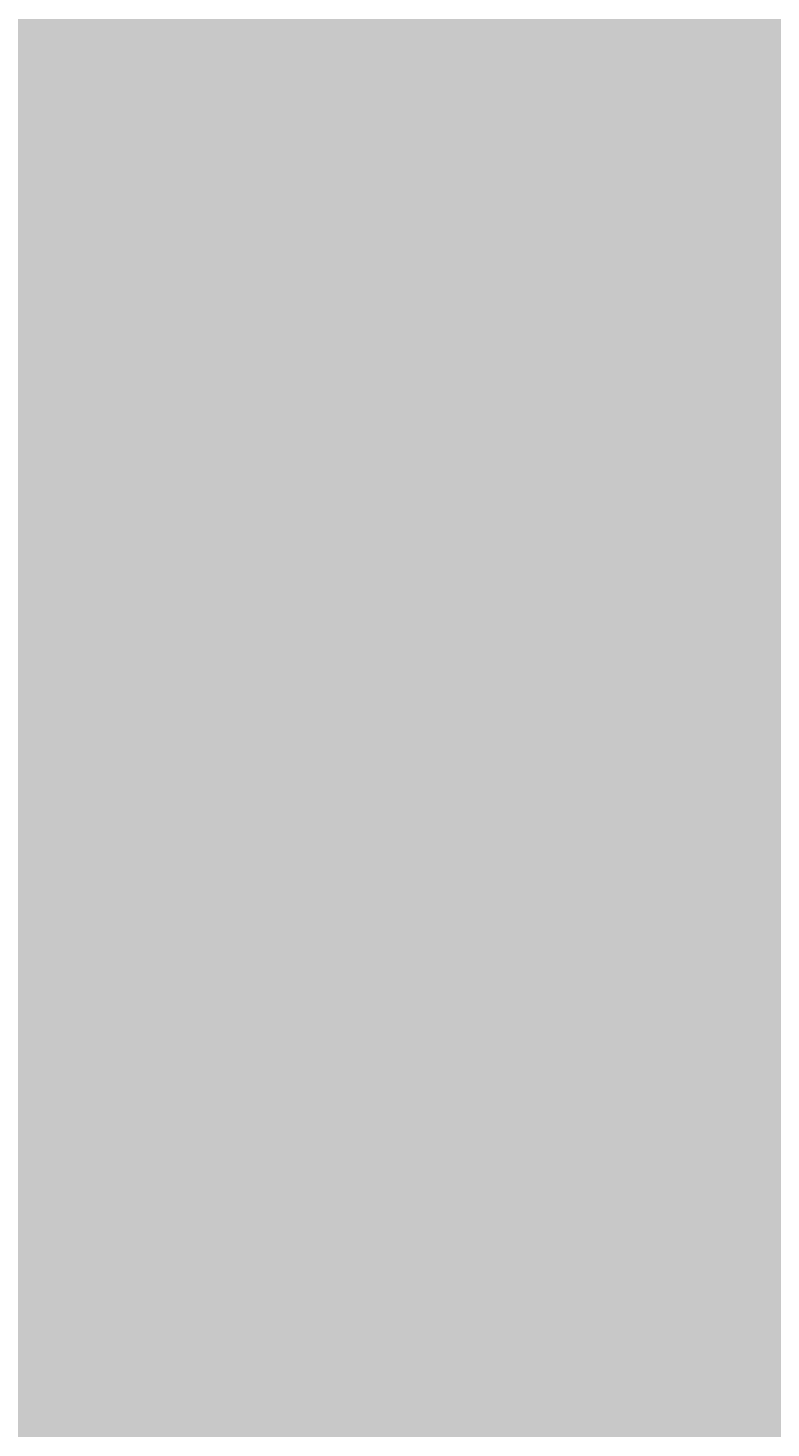
# Model space of a CAD drawing. Units: millimetres. Extents: x -22994 to 29398, y -19990 to 20176.
# Tile 125 of 135: x 391 to 480, y 5 to 173. Entities that reach past the tile are written whole.
import ezdxf

# ---------------------------------------------------------------- set-up
doc = ezdxf.new("R2010")
doc.units = ezdxf.units.MM
doc.header["$MEASUREMENT"] = 0
doc.layers.add('M-DIMS', color=2, linetype='Continuous', lineweight=18)
doc.styles.get("Standard").update_dxf_attribs({"font": 'arial.ttf'})
doc.dimstyles.get("Standard").update_dxf_attribs({"dimtxt": 0.18, "dimasz": 10000, "dimexe": 0.18, "dimexo": 0.0625, "dimgap": 0.09, "dimtad": 0, "dimtih": 1, "dimtoh": 1, "dimdec": 0, "dimzin": 0, "dimdsep": 46, "dimtxsty": 'Standard', "dimcen": 0.09, "dimadec": 0, "dimazin": 0, "dimtfac": 1, "dimtdec": 0, "dimtofl": 0, "dimtmove": 0, "dimatfit": 3, "dimfxl": 1, "dimtolj": 1, "dimtzin": 0, "dimlwd": 30, "dimarcsym": 0})

# ---------------------------------------------------------------- blocks, each defined once
blk = doc.blocks.new('*D2')
at = {"layer": 'Defpoints', "color": 0, "transparency": 16777216}
for p in [(6.68, 10.27), (290.85, 10.27), (290.85, -5.08)]:
    blk.add_point(p, dxfattribs=at)
at = {"layer": 'M-DIMS', "color": 0, "lineweight": -2, "transparency": 16777216}
for p, q in [((6.68, 10.21), (6.68, -5.26)), ((290.85, 10.21), (290.85, -5.26))]:
    blk.add_line(p, q, dxfattribs=at)
at = {"layer": 'M-DIMS', "color": 0, "lineweight": 30, "transparency": 16777216}
for p, q in [((-9993.32, -5.08), (-19993.32, -5.08)), ((10290.85, -5.08), (20290.85, -5.08))]:
    blk.add_line(p, q, dxfattribs=at)
at = {"layer": 'M-DIMS', "color": 0, "transparency": 16777216}
for points in [[(-9993.32, 1661.59), (-9993.32, -1671.75), (6.68, -5.08)], [(10290.85, 1661.59), (10290.85, -1671.75), (290.85, -5.08)]]:
    blk.add_solid(points, dxfattribs=at)
at = {"layer": 'M-DIMS', "color": 0, "transparency": 16777216, "insert": (148.76, -5.08), "char_height": 0.18, "attachment_point": 5}
blk.add_mtext('\\A1;284.2', dxfattribs=at)
blk = doc.blocks.new('*D3')
at = {"layer": 'Defpoints', "color": 0, "transparency": 16777216}
for p in [(110.26, 204.17), (110.26, 176.37), (95.83, 127.97)]:
    blk.add_point(p, dxfattribs=at)
at = {"layer": 'M-DIMS', "color": 0, "lineweight": 30, "transparency": 16777216}
for p, q in [((-9904.17, 204.17), (-19904.17, 204.17)), ((10110.26, 204.17), (20110.26, 204.17))]:
    blk.add_line(p, q, dxfattribs=at)
at = {"layer": 'M-DIMS', "color": 0, "lineweight": -2, "transparency": 16777216}
for p, q in [((95.83, 128.03), (95.83, 204.35)), ((110.26, 176.43), (110.26, 204.35))]:
    blk.add_line(p, q, dxfattribs=at)
at = {"layer": 'M-DIMS', "color": 0, "transparency": 16777216}
for points in [[(-9904.17, 1870.83), (-9904.17, -1462.5), (95.83, 204.17)], [(10110.26, 1870.83), (10110.26, -1462.5), (110.26, 204.17)]]:
    blk.add_solid(points, dxfattribs=at)
at = {"layer": 'M-DIMS', "color": 0, "transparency": 16777216, "insert": (103.05, 204.17), "char_height": 0.18, "attachment_point": 5}
blk.add_mtext('\\A1;14.432', dxfattribs=at)
blk = doc.blocks.new('*D4')
at = {"layer": 'Defpoints', "color": 0, "transparency": 16777216}
for p in [(116.26, 204.17), (110.26, 176.37), (116.26, 176.37)]:
    blk.add_point(p, dxfattribs=at)
at = {"layer": 'M-DIMS', "color": 0, "lineweight": 30, "transparency": 16777216}
for p, q in [((-9889.74, 204.17), (-19889.74, 204.17)), ((10116.26, 204.17), (20116.26, 204.17))]:
    blk.add_line(p, q, dxfattribs=at)
at = {"layer": 'M-DIMS', "color": 0, "lineweight": -2, "transparency": 16777216}
for p, q in [((110.26, 176.43), (110.26, 204.35)), ((116.26, 176.43), (116.26, 204.35))]:
    blk.add_line(p, q, dxfattribs=at)
at = {"layer": 'M-DIMS', "color": 0, "transparency": 16777216}
for points in [[(-9889.74, 1870.83), (-9889.74, -1462.5), (110.26, 204.17)], [(10116.26, 1870.83), (10116.26, -1462.5), (116.26, 204.17)]]:
    blk.add_solid(points, dxfattribs=at)
at = {"layer": 'M-DIMS', "color": 0, "transparency": 16777216, "insert": (113.26, 204.17), "char_height": 0.18, "attachment_point": 5}
blk.add_mtext('\\A1;6', dxfattribs=at)
blk = doc.blocks.new('*D5')
at = {"layer": 'Defpoints', "color": 0, "transparency": 16777216}
for p in [(181.26, 204.17), (116.26, 176.37), (181.26, 176.37)]:
    blk.add_point(p, dxfattribs=at)
at = {"layer": 'M-DIMS', "color": 0, "lineweight": 30, "transparency": 16777216}
for p, q in [((-9883.74, 204.17), (-19883.74, 204.17)), ((10181.26, 204.17), (20181.26, 204.17))]:
    blk.add_line(p, q, dxfattribs=at)
at = {"layer": 'M-DIMS', "color": 0, "lineweight": -2, "transparency": 16777216}
for p, q in [((116.26, 176.43), (116.26, 204.35)), ((181.26, 176.43), (181.26, 204.35))]:
    blk.add_line(p, q, dxfattribs=at)
at = {"layer": 'M-DIMS', "color": 0, "transparency": 16777216}
for points in [[(-9883.74, 1870.83), (-9883.74, -1462.5), (116.26, 204.17)], [(10181.26, 1870.83), (10181.26, -1462.5), (181.26, 204.17)]]:
    blk.add_solid(points, dxfattribs=at)
at = {"layer": 'M-DIMS', "color": 0, "transparency": 16777216, "insert": (148.76, 204.17), "char_height": 0.18, "attachment_point": 5}
blk.add_mtext('\\A1;65', dxfattribs=at)
blk = doc.blocks.new('*D6')
at = {"layer": 'Defpoints', "color": 0, "transparency": 16777216}
for p in [(187.26, 204.17), (181.26, 176.37), (187.26, 176.37)]:
    blk.add_point(p, dxfattribs=at)
at = {"layer": 'M-DIMS', "color": 0, "lineweight": 30, "transparency": 16777216}
for p, q in [((-9818.74, 204.17), (-19818.74, 204.17)), ((10187.26, 204.17), (20187.26, 204.17))]:
    blk.add_line(p, q, dxfattribs=at)
at = {"layer": 'M-DIMS', "color": 0, "lineweight": -2, "transparency": 16777216}
for p, q in [((181.26, 176.43), (181.26, 204.35)), ((187.26, 176.43), (187.26, 204.35))]:
    blk.add_line(p, q, dxfattribs=at)
at = {"layer": 'M-DIMS', "color": 0, "transparency": 16777216}
for points in [[(-9818.74, 1870.83), (-9818.74, -1462.5), (181.26, 204.17)], [(10187.26, 1870.83), (10187.26, -1462.5), (187.26, 204.17)]]:
    blk.add_solid(points, dxfattribs=at)
at = {"layer": 'M-DIMS', "color": 0, "transparency": 16777216, "insert": (184.26, 204.17), "char_height": 0.18, "attachment_point": 5}
blk.add_mtext('\\A1;6', dxfattribs=at)
blk = doc.blocks.new('*D7')
at = {"layer": 'Defpoints', "color": 0, "transparency": 16777216}
for p in [(201.7, 204.17), (187.26, 176.37), (201.7, 127.97)]:
    blk.add_point(p, dxfattribs=at)
at = {"layer": 'M-DIMS', "color": 0, "lineweight": 30, "transparency": 16777216}
for p, q in [((-9812.74, 204.17), (-19812.74, 204.17)), ((10201.7, 204.17), (20201.7, 204.17))]:
    blk.add_line(p, q, dxfattribs=at)
at = {"layer": 'M-DIMS', "color": 0, "lineweight": -2, "transparency": 16777216}
for p, q in [((187.26, 176.43), (187.26, 204.35)), ((201.7, 128.03), (201.7, 204.35))]:
    blk.add_line(p, q, dxfattribs=at)
at = {"layer": 'M-DIMS', "color": 0, "transparency": 16777216}
for points in [[(-9812.74, 1870.83), (-9812.74, -1462.5), (187.26, 204.17)], [(10201.7, 1870.83), (10201.7, -1462.5), (201.7, 204.17)]]:
    blk.add_solid(points, dxfattribs=at)
at = {"layer": 'M-DIMS', "color": 0, "transparency": 16777216, "insert": (194.48, 204.17), "char_height": 0.18, "attachment_point": 5}
blk.add_mtext('\\A1;14.432', dxfattribs=at)
blk = doc.blocks.new('*D8')
at = {"layer": 'Defpoints', "color": 0, "transparency": 16777216}
for p in [(227.65, 204.17), (227.65, 146.73), (201.7, 127.97)]:
    blk.add_point(p, dxfattribs=at)
at = {"layer": 'M-DIMS', "color": 0, "lineweight": 30, "transparency": 16777216}
for p, q in [((-9798.3, 204.17), (-19798.3, 204.17)), ((10227.65, 204.17), (20227.65, 204.17))]:
    blk.add_line(p, q, dxfattribs=at)
at = {"layer": 'M-DIMS', "color": 0, "lineweight": -2, "transparency": 16777216}
for p, q in [((201.7, 128.03), (201.7, 204.35)), ((227.65, 146.79), (227.65, 204.35))]:
    blk.add_line(p, q, dxfattribs=at)
at = {"layer": 'M-DIMS', "color": 0, "transparency": 16777216}
for points in [[(-9798.3, 1870.83), (-9798.3, -1462.5), (201.7, 204.17)], [(10227.65, 1870.83), (10227.65, -1462.5), (227.65, 204.17)]]:
    blk.add_solid(points, dxfattribs=at)
at = {"layer": 'M-DIMS', "color": 0, "transparency": 16777216, "insert": (214.67, 204.17), "char_height": 0.18, "attachment_point": 5}
blk.add_mtext('\\A1;25.95', dxfattribs=at)
blk = doc.blocks.new('*D9')
at = {"layer": 'Defpoints', "color": 0, "transparency": 16777216}
for p in [(187.26, 176.37), (306.2, 176.37), (290.85, 10.27)]:
    blk.add_point(p, dxfattribs=at)
at = {"layer": 'M-DIMS', "color": 0, "lineweight": 30, "transparency": 16777216}
for p, q in [((306.2, 10176.37), (306.2, 20176.37)), ((306.2, -9989.73), (306.2, -19989.73))]:
    blk.add_line(p, q, dxfattribs=at)
at = {"layer": 'M-DIMS', "color": 0, "lineweight": -2, "transparency": 16777216}
for p, q in [((187.33, 176.37), (306.38, 176.37)), ((290.91, 10.27), (306.38, 10.27))]:
    blk.add_line(p, q, dxfattribs=at)
at = {"layer": 'M-DIMS', "color": 0, "transparency": 16777216}
for points in [[(-1360.46, 10176.37), (1972.87, 10176.37), (306.2, 176.37)], [(-1360.46, -9989.73), (1972.87, -9989.73), (306.2, 10.27)]]:
    blk.add_solid(points, dxfattribs=at)
at = {"layer": 'M-DIMS', "color": 0, "transparency": 16777216, "insert": (306.2, 93.32), "char_height": 0.18, "attachment_point": 5}
blk.add_mtext('\\A1;166.1', dxfattribs=at)
blk = doc.blocks.new('*D10')
at = {"layer": 'Defpoints', "color": 0, "transparency": 16777216}
for p in [(125.65, 136.07), (133.35, 136.07), (133.35, -5.08)]:
    blk.add_point(p, dxfattribs=at)
at = {"layer": 'M-DIMS', "color": 0, "lineweight": -2, "transparency": 16777216}
for p, q in [((125.65, 136.01), (125.65, -5.26)), ((133.35, 136.01), (133.35, -5.26))]:
    blk.add_line(p, q, dxfattribs=at)
at = {"layer": 'M-DIMS', "color": 0, "lineweight": 30, "transparency": 16777216}
for p, q in [((-9874.35, -5.08), (-19874.35, -5.08)), ((10133.35, -5.08), (20133.35, -5.08))]:
    blk.add_line(p, q, dxfattribs=at)
at = {"layer": 'M-DIMS', "color": 0, "transparency": 16777216}
for points in [[(-9874.35, 1661.59), (-9874.35, -1671.75), (125.65, -5.08)], [(10133.35, 1661.59), (10133.35, -1671.75), (133.35, -5.08)]]:
    blk.add_solid(points, dxfattribs=at)
at = {"layer": 'M-DIMS', "color": 0, "transparency": 16777216, "insert": (129.5, -5.08), "char_height": 0.18, "attachment_point": 5}
blk.add_mtext('\\A1;7.696', dxfattribs=at)
blk = doc.blocks.new('*D11')
at = {"layer": 'Defpoints', "color": 0, "transparency": 16777216}
for p in [(133.35, 136.07), (135.65, 136.07), (135.65, -5.08)]:
    blk.add_point(p, dxfattribs=at)
at = {"layer": 'M-DIMS', "color": 0, "lineweight": -2, "transparency": 16777216}
for p, q in [((133.35, 136.01), (133.35, -5.26)), ((135.65, 136.01), (135.65, -5.26))]:
    blk.add_line(p, q, dxfattribs=at)
at = {"layer": 'M-DIMS', "color": 0, "lineweight": 30, "transparency": 16777216}
for p, q in [((-9866.65, -5.08), (-19866.65, -5.08)), ((10135.65, -5.08), (20135.65, -5.08))]:
    blk.add_line(p, q, dxfattribs=at)
at = {"layer": 'M-DIMS', "color": 0, "transparency": 16777216}
for points in [[(-9866.65, 1661.59), (-9866.65, -1671.75), (133.35, -5.08)], [(10135.65, 1661.59), (10135.65, -1671.75), (135.65, -5.08)]]:
    blk.add_solid(points, dxfattribs=at)
at = {"layer": 'M-DIMS', "color": 0, "transparency": 16777216, "insert": (134.5, -5.08), "char_height": 0.18, "attachment_point": 5}
blk.add_mtext('\\A1;2.304', dxfattribs=at)
blk = doc.blocks.new('*D12')
at = {"layer": 'Defpoints', "color": 0, "transparency": 16777216}
for p in [(135.65, 136.07), (145.65, 136.07), (145.65, -5.08)]:
    blk.add_point(p, dxfattribs=at)
at = {"layer": 'M-DIMS', "color": 0, "lineweight": -2, "transparency": 16777216}
for p, q in [((135.65, 136.01), (135.65, -5.26)), ((145.65, 136.01), (145.65, -5.26))]:
    blk.add_line(p, q, dxfattribs=at)
at = {"layer": 'M-DIMS', "color": 0, "lineweight": 30, "transparency": 16777216}
for p, q in [((-9864.35, -5.08), (-19864.35, -5.08)), ((10145.65, -5.08), (20145.65, -5.08))]:
    blk.add_line(p, q, dxfattribs=at)
at = {"layer": 'M-DIMS', "color": 0, "transparency": 16777216}
for points in [[(-9864.35, 1661.59), (-9864.35, -1671.75), (135.65, -5.08)], [(10145.65, 1661.59), (10145.65, -1671.75), (145.65, -5.08)]]:
    blk.add_solid(points, dxfattribs=at)
at = {"layer": 'M-DIMS', "color": 0, "transparency": 16777216, "insert": (140.65, -5.08), "char_height": 0.18, "attachment_point": 5}
blk.add_mtext('\\A1;10', dxfattribs=at)
blk = doc.blocks.new('*D13')
at = {"layer": 'Defpoints', "color": 0, "transparency": 16777216}
for p in [(145.65, 136.07), (155.65, 136.07), (155.65, -5.08)]:
    blk.add_point(p, dxfattribs=at)
at = {"layer": 'M-DIMS', "color": 0, "lineweight": -2, "transparency": 16777216}
for p, q in [((145.65, 136.01), (145.65, -5.26)), ((155.65, 136.01), (155.65, -5.26))]:
    blk.add_line(p, q, dxfattribs=at)
at = {"layer": 'M-DIMS', "color": 0, "lineweight": 30, "transparency": 16777216}
for p, q in [((-9854.35, -5.08), (-19854.35, -5.08)), ((10155.65, -5.08), (20155.65, -5.08))]:
    blk.add_line(p, q, dxfattribs=at)
at = {"layer": 'M-DIMS', "color": 0, "transparency": 16777216}
for points in [[(-9854.35, 1661.59), (-9854.35, -1671.75), (145.65, -5.08)], [(10155.65, 1661.59), (10155.65, -1671.75), (155.65, -5.08)]]:
    blk.add_solid(points, dxfattribs=at)
at = {"layer": 'M-DIMS', "color": 0, "transparency": 16777216, "insert": (150.65, -5.08), "char_height": 0.18, "attachment_point": 5}
blk.add_mtext('\\A1;10', dxfattribs=at)
blk = doc.blocks.new('*D14')
at = {"layer": 'Defpoints', "color": 0, "transparency": 16777216}
for p in [(155.65, 136.07), (165.65, 136.07), (165.65, -5.08)]:
    blk.add_point(p, dxfattribs=at)
at = {"layer": 'M-DIMS', "color": 0, "lineweight": -2, "transparency": 16777216}
for p, q in [((155.65, 136.01), (155.65, -5.26)), ((165.65, 136.01), (165.65, -5.26))]:
    blk.add_line(p, q, dxfattribs=at)
at = {"layer": 'M-DIMS', "color": 0, "lineweight": 30, "transparency": 16777216}
for p, q in [((-9844.35, -5.08), (-19844.35, -5.08)), ((10165.65, -5.08), (20165.65, -5.08))]:
    blk.add_line(p, q, dxfattribs=at)
at = {"layer": 'M-DIMS', "color": 0, "transparency": 16777216}
for points in [[(-9844.35, 1661.59), (-9844.35, -1671.75), (155.65, -5.08)], [(10165.65, 1661.59), (10165.65, -1671.75), (165.65, -5.08)]]:
    blk.add_solid(points, dxfattribs=at)
at = {"layer": 'M-DIMS', "color": 0, "transparency": 16777216, "insert": (160.65, -5.08), "char_height": 0.18, "attachment_point": 5}
blk.add_mtext('\\A1;10', dxfattribs=at)
blk = doc.blocks.new('*D15')
at = {"layer": 'Defpoints', "color": 0, "transparency": 16777216}
for p in [(173.35, 154.79), (173.35, 136.07), (306.2, 136.07)]:
    blk.add_point(p, dxfattribs=at)
at = {"layer": 'M-DIMS', "color": 0, "lineweight": 30, "transparency": 16777216}
for p, q in [((306.2, 10154.79), (306.2, 20154.79)), ((306.2, -9863.93), (306.2, -19863.93))]:
    blk.add_line(p, q, dxfattribs=at)
at = {"layer": 'M-DIMS', "color": 0, "lineweight": -2, "transparency": 16777216}
for p, q in [((173.41, 154.79), (306.38, 154.79)), ((173.41, 136.07), (306.38, 136.07))]:
    blk.add_line(p, q, dxfattribs=at)
at = {"layer": 'M-DIMS', "color": 0, "transparency": 16777216}
for points in [[(-1360.46, 10154.79), (1972.87, 10154.79), (306.2, 154.79)], [(-1360.46, -9863.93), (1972.87, -9863.93), (306.2, 136.07)]]:
    blk.add_solid(points, dxfattribs=at)
at = {"layer": 'M-DIMS', "color": 0, "transparency": 16777216, "insert": (306.2, 145.43), "char_height": 0.18, "attachment_point": 5}
blk.add_mtext('\\A1;18.717', dxfattribs=at)
blk = doc.blocks.new('*D16')
at = {"layer": 'Defpoints', "color": 0, "transparency": 16777216}
for p in [(120.17, 204.17), (110.47, 48.03), (120.17, 48.03)]:
    blk.add_point(p, dxfattribs=at)
at = {"layer": 'M-DIMS', "color": 0, "lineweight": 30, "transparency": 16777216}
for p, q in [((-9889.53, 204.17), (-19889.53, 204.17)), ((10120.17, 204.17), (20120.17, 204.17))]:
    blk.add_line(p, q, dxfattribs=at)
at = {"layer": 'M-DIMS', "color": 0, "lineweight": -2, "transparency": 16777216}
for p, q in [((110.47, 48.1), (110.47, 204.35)), ((120.17, 48.1), (120.17, 204.35))]:
    blk.add_line(p, q, dxfattribs=at)
at = {"layer": 'M-DIMS', "color": 0, "transparency": 16777216}
for points in [[(-9889.53, 1870.83), (-9889.53, -1462.5), (110.47, 204.17)], [(10120.17, 1870.83), (10120.17, -1462.5), (120.17, 204.17)]]:
    blk.add_solid(points, dxfattribs=at)
at = {"layer": 'M-DIMS', "color": 0, "transparency": 16777216, "insert": (115.32, 204.17), "char_height": 0.18, "attachment_point": 5}
blk.add_mtext('\\A1;9.704', dxfattribs=at)
blk = doc.blocks.new('*D17')
at = {"layer": 'Defpoints', "color": 0, "transparency": 16777216}
for p in [(126.17, 204.17), (120.17, 48.03), (126.17, 48.03)]:
    blk.add_point(p, dxfattribs=at)
at = {"layer": 'M-DIMS', "color": 0, "lineweight": 30, "transparency": 16777216}
for p, q in [((-9879.83, 204.17), (-19879.83, 204.17)), ((10126.17, 204.17), (20126.17, 204.17))]:
    blk.add_line(p, q, dxfattribs=at)
at = {"layer": 'M-DIMS', "color": 0, "lineweight": -2, "transparency": 16777216}
for p, q in [((120.17, 48.1), (120.17, 204.35)), ((126.17, 48.1), (126.17, 204.35))]:
    blk.add_line(p, q, dxfattribs=at)
at = {"layer": 'M-DIMS', "color": 0, "transparency": 16777216}
for points in [[(-9879.83, 1870.83), (-9879.83, -1462.5), (120.17, 204.17)], [(10126.17, 1870.83), (10126.17, -1462.5), (126.17, 204.17)]]:
    blk.add_solid(points, dxfattribs=at)
at = {"layer": 'M-DIMS', "color": 0, "transparency": 16777216, "insert": (123.17, 204.17), "char_height": 0.18, "attachment_point": 5}
blk.add_mtext('\\A1;6', dxfattribs=at)
blk = doc.blocks.new('*D18')
at = {"layer": 'Defpoints', "color": 0, "transparency": 16777216}
for p in [(132.17, 204.17), (126.17, 48.03), (132.17, 48.03)]:
    blk.add_point(p, dxfattribs=at)
at = {"layer": 'M-DIMS', "color": 0, "lineweight": 30, "transparency": 16777216}
for p, q in [((-9873.83, 204.17), (-19873.83, 204.17)), ((10132.17, 204.17), (20132.17, 204.17))]:
    blk.add_line(p, q, dxfattribs=at)
at = {"layer": 'M-DIMS', "color": 0, "lineweight": -2, "transparency": 16777216}
for p, q in [((126.17, 48.1), (126.17, 204.35)), ((132.17, 48.1), (132.17, 204.35))]:
    blk.add_line(p, q, dxfattribs=at)
at = {"layer": 'M-DIMS', "color": 0, "transparency": 16777216}
for points in [[(-9873.83, 1870.83), (-9873.83, -1462.5), (126.17, 204.17)], [(10132.17, 1870.83), (10132.17, -1462.5), (132.17, 204.17)]]:
    blk.add_solid(points, dxfattribs=at)
at = {"layer": 'M-DIMS', "color": 0, "transparency": 16777216, "insert": (129.17, 204.17), "char_height": 0.18, "attachment_point": 5}
blk.add_mtext('\\A1;6', dxfattribs=at)
blk = doc.blocks.new('*D19')
at = {"layer": 'Defpoints', "color": 0, "transparency": 16777216}
for p in [(138.17, 204.17), (132.17, 48.03), (138.17, 48.03)]:
    blk.add_point(p, dxfattribs=at)
at = {"layer": 'M-DIMS', "color": 0, "lineweight": 30, "transparency": 16777216}
for p, q in [((-9867.83, 204.17), (-19867.83, 204.17)), ((10138.17, 204.17), (20138.17, 204.17))]:
    blk.add_line(p, q, dxfattribs=at)
at = {"layer": 'M-DIMS', "color": 0, "lineweight": -2, "transparency": 16777216}
for p, q in [((132.17, 48.1), (132.17, 204.35)), ((138.17, 48.1), (138.17, 204.35))]:
    blk.add_line(p, q, dxfattribs=at)
at = {"layer": 'M-DIMS', "color": 0, "transparency": 16777216}
for points in [[(-9867.83, 1870.83), (-9867.83, -1462.5), (132.17, 204.17)], [(10138.17, 1870.83), (10138.17, -1462.5), (138.17, 204.17)]]:
    blk.add_solid(points, dxfattribs=at)
at = {"layer": 'M-DIMS', "color": 0, "transparency": 16777216, "insert": (135.17, 204.17), "char_height": 0.18, "attachment_point": 5}
blk.add_mtext('\\A1;6', dxfattribs=at)
blk = doc.blocks.new('*D20')
at = {"layer": 'Defpoints', "color": 0, "transparency": 16777216}
for p in [(144.17, 204.17), (138.17, 48.03), (144.17, 48.03)]:
    blk.add_point(p, dxfattribs=at)
at = {"layer": 'M-DIMS', "color": 0, "lineweight": 30, "transparency": 16777216}
for p, q in [((-9861.83, 204.17), (-19861.83, 204.17)), ((10144.17, 204.17), (20144.17, 204.17))]:
    blk.add_line(p, q, dxfattribs=at)
at = {"layer": 'M-DIMS', "color": 0, "lineweight": -2, "transparency": 16777216}
for p, q in [((138.17, 48.1), (138.17, 204.35)), ((144.17, 48.1), (144.17, 204.35))]:
    blk.add_line(p, q, dxfattribs=at)
at = {"layer": 'M-DIMS', "color": 0, "transparency": 16777216}
for points in [[(-9861.83, 1870.83), (-9861.83, -1462.5), (138.17, 204.17)], [(10144.17, 1870.83), (10144.17, -1462.5), (144.17, 204.17)]]:
    blk.add_solid(points, dxfattribs=at)
at = {"layer": 'M-DIMS', "color": 0, "transparency": 16777216, "insert": (141.17, 204.17), "char_height": 0.18, "attachment_point": 5}
blk.add_mtext('\\A1;6', dxfattribs=at)
blk = doc.blocks.new('*D21')
at = {"layer": 'Defpoints', "color": 0, "transparency": 16777216}
for p in [(149.12, 204.17), (144.17, 48.03), (149.12, 48.03)]:
    blk.add_point(p, dxfattribs=at)
at = {"layer": 'M-DIMS', "color": 0, "lineweight": 30, "transparency": 16777216}
for p, q in [((-9855.83, 204.17), (-19855.83, 204.17)), ((10149.12, 204.17), (20149.12, 204.17))]:
    blk.add_line(p, q, dxfattribs=at)
at = {"layer": 'M-DIMS', "color": 0, "lineweight": -2, "transparency": 16777216}
for p, q in [((144.17, 48.1), (144.17, 204.35)), ((149.12, 48.1), (149.12, 204.35))]:
    blk.add_line(p, q, dxfattribs=at)
at = {"layer": 'M-DIMS', "color": 0, "transparency": 16777216}
for points in [[(-9855.83, 1870.83), (-9855.83, -1462.5), (144.17, 204.17)], [(10149.12, 1870.83), (10149.12, -1462.5), (149.12, 204.17)]]:
    blk.add_solid(points, dxfattribs=at)
at = {"layer": 'M-DIMS', "color": 0, "transparency": 16777216, "insert": (146.64, 204.17), "char_height": 0.18, "attachment_point": 5}
blk.add_mtext('\\A1;4.945', dxfattribs=at)
blk = doc.blocks.new('*D22')
at = {"layer": 'Defpoints', "color": 0, "transparency": 16777216}
for p in [(149.12, 30.99), (155.12, 30.99), (155.12, -5.08)]:
    blk.add_point(p, dxfattribs=at)
at = {"layer": 'M-DIMS', "color": 0, "lineweight": -2, "transparency": 16777216}
for p, q in [((149.12, 30.93), (149.12, -5.26)), ((155.12, 30.93), (155.12, -5.26))]:
    blk.add_line(p, q, dxfattribs=at)
at = {"layer": 'M-DIMS', "color": 0, "lineweight": 30, "transparency": 16777216}
for p, q in [((-9850.88, -5.08), (-19850.88, -5.08)), ((10155.12, -5.08), (20155.12, -5.08))]:
    blk.add_line(p, q, dxfattribs=at)
at = {"layer": 'M-DIMS', "color": 0, "transparency": 16777216}
for points in [[(-9850.88, 1661.59), (-9850.88, -1671.75), (149.12, -5.08)], [(10155.12, 1661.59), (10155.12, -1671.75), (155.12, -5.08)]]:
    blk.add_solid(points, dxfattribs=at)
at = {"layer": 'M-DIMS', "color": 0, "transparency": 16777216, "insert": (152.12, -5.08), "char_height": 0.18, "attachment_point": 5}
blk.add_mtext('\\A1;6', dxfattribs=at)
blk = doc.blocks.new('*D23')
at = {"layer": 'Defpoints', "color": 0, "transparency": 16777216}
for p in [(155.12, 30.99), (161.12, 30.99), (161.12, -5.08)]:
    blk.add_point(p, dxfattribs=at)
at = {"layer": 'M-DIMS', "color": 0, "lineweight": -2, "transparency": 16777216}
for p, q in [((155.12, 30.93), (155.12, -5.26)), ((161.12, 30.93), (161.12, -5.26))]:
    blk.add_line(p, q, dxfattribs=at)
at = {"layer": 'M-DIMS', "color": 0, "lineweight": 30, "transparency": 16777216}
for p, q in [((-9844.88, -5.08), (-19844.88, -5.08)), ((10161.12, -5.08), (20161.12, -5.08))]:
    blk.add_line(p, q, dxfattribs=at)
at = {"layer": 'M-DIMS', "color": 0, "transparency": 16777216}
for points in [[(-9844.88, 1661.59), (-9844.88, -1671.75), (155.12, -5.08)], [(10161.12, 1661.59), (10161.12, -1671.75), (161.12, -5.08)]]:
    blk.add_solid(points, dxfattribs=at)
at = {"layer": 'M-DIMS', "color": 0, "transparency": 16777216, "insert": (158.12, -5.08), "char_height": 0.18, "attachment_point": 5}
blk.add_mtext('\\A1;6', dxfattribs=at)
blk = doc.blocks.new('*D24')
at = {"layer": 'Defpoints', "color": 0, "transparency": 16777216}
for p in [(161.12, 30.99), (166.44, 30.99), (166.44, -5.08)]:
    blk.add_point(p, dxfattribs=at)
at = {"layer": 'M-DIMS', "color": 0, "lineweight": -2, "transparency": 16777216}
for p, q in [((161.12, 30.93), (161.12, -5.26)), ((166.44, 30.93), (166.44, -5.26))]:
    blk.add_line(p, q, dxfattribs=at)
at = {"layer": 'M-DIMS', "color": 0, "lineweight": 30, "transparency": 16777216}
for p, q in [((-9838.88, -5.08), (-19838.88, -5.08)), ((10166.44, -5.08), (20166.44, -5.08))]:
    blk.add_line(p, q, dxfattribs=at)
at = {"layer": 'M-DIMS', "color": 0, "transparency": 16777216}
for points in [[(-9838.88, 1661.59), (-9838.88, -1671.75), (161.12, -5.08)], [(10166.44, 1661.59), (10166.44, -1671.75), (166.44, -5.08)]]:
    blk.add_solid(points, dxfattribs=at)
at = {"layer": 'M-DIMS', "color": 0, "transparency": 16777216, "insert": (163.78, -5.08), "char_height": 0.18, "attachment_point": 5}
blk.add_mtext('\\A1;5.323', dxfattribs=at)
blk = doc.blocks.new('*D25')
at = {"layer": 'Defpoints', "color": 0, "transparency": 16777216}
for p in [(166.44, 30.99), (172.44, 30.99), (172.44, -5.08)]:
    blk.add_point(p, dxfattribs=at)
at = {"layer": 'M-DIMS', "color": 0, "lineweight": -2, "transparency": 16777216}
for p, q in [((166.44, 30.93), (166.44, -5.26)), ((172.44, 30.93), (172.44, -5.26))]:
    blk.add_line(p, q, dxfattribs=at)
at = {"layer": 'M-DIMS', "color": 0, "lineweight": 30, "transparency": 16777216}
for p, q in [((-9833.56, -5.08), (-19833.56, -5.08)), ((10172.44, -5.08), (20172.44, -5.08))]:
    blk.add_line(p, q, dxfattribs=at)
at = {"layer": 'M-DIMS', "color": 0, "transparency": 16777216}
for points in [[(-9833.56, 1661.59), (-9833.56, -1671.75), (166.44, -5.08)], [(10172.44, 1661.59), (10172.44, -1671.75), (172.44, -5.08)]]:
    blk.add_solid(points, dxfattribs=at)
at = {"layer": 'M-DIMS', "color": 0, "transparency": 16777216, "insert": (169.44, -5.08), "char_height": 0.18, "attachment_point": 5}
blk.add_mtext('\\A1;6', dxfattribs=at)
blk = doc.blocks.new('*D26')
at = {"layer": 'Defpoints', "color": 0, "transparency": 16777216}
for p in [(172.44, 30.99), (178.44, 30.99), (178.44, -5.08)]:
    blk.add_point(p, dxfattribs=at)
at = {"layer": 'M-DIMS', "color": 0, "lineweight": -2, "transparency": 16777216}
for p, q in [((172.44, 30.93), (172.44, -5.26)), ((178.44, 30.93), (178.44, -5.26))]:
    blk.add_line(p, q, dxfattribs=at)
at = {"layer": 'M-DIMS', "color": 0, "lineweight": 30, "transparency": 16777216}
for p, q in [((-9827.56, -5.08), (-19827.56, -5.08)), ((10178.44, -5.08), (20178.44, -5.08))]:
    blk.add_line(p, q, dxfattribs=at)
at = {"layer": 'M-DIMS', "color": 0, "transparency": 16777216}
for points in [[(-9827.56, 1661.59), (-9827.56, -1671.75), (172.44, -5.08)], [(10178.44, 1661.59), (10178.44, -1671.75), (178.44, -5.08)]]:
    blk.add_solid(points, dxfattribs=at)
at = {"layer": 'M-DIMS', "color": 0, "transparency": 16777216, "insert": (175.44, -5.08), "char_height": 0.18, "attachment_point": 5}
blk.add_mtext('\\A1;6', dxfattribs=at)
blk = doc.blocks.new('*D27')
at = {"layer": 'Defpoints', "color": 0, "transparency": 16777216}
for p in [(178.44, 30.99), (188.12, 30.99), (188.12, -5.08)]:
    blk.add_point(p, dxfattribs=at)
at = {"layer": 'M-DIMS', "color": 0, "lineweight": -2, "transparency": 16777216}
for p, q in [((178.44, 30.93), (178.44, -5.26)), ((188.12, 30.93), (188.12, -5.26))]:
    blk.add_line(p, q, dxfattribs=at)
at = {"layer": 'M-DIMS', "color": 0, "lineweight": 30, "transparency": 16777216}
for p, q in [((-9821.56, -5.08), (-19821.56, -5.08)), ((10188.12, -5.08), (20188.12, -5.08))]:
    blk.add_line(p, q, dxfattribs=at)
at = {"layer": 'M-DIMS', "color": 0, "transparency": 16777216}
for points in [[(-9821.56, 1661.59), (-9821.56, -1671.75), (178.44, -5.08)], [(10188.12, 1661.59), (10188.12, -1671.75), (188.12, -5.08)]]:
    blk.add_solid(points, dxfattribs=at)
at = {"layer": 'M-DIMS', "color": 0, "transparency": 16777216, "insert": (183.28, -5.08), "char_height": 0.18, "attachment_point": 5}
blk.add_mtext('\\A1;9.679', dxfattribs=at)
blk = doc.blocks.new('*D28')
at = {"layer": 'Defpoints', "color": 0, "transparency": 16777216}
for p in [(188.12, 48.03), (306.2, 48.03), (188.12, 30.99)]:
    blk.add_point(p, dxfattribs=at)
at = {"layer": 'M-DIMS', "color": 0, "lineweight": 30, "transparency": 16777216}
for p, q in [((306.2, 10048.03), (306.2, 20048.03)), ((306.2, -9969.01), (306.2, -19969.01))]:
    blk.add_line(p, q, dxfattribs=at)
at = {"layer": 'M-DIMS', "color": 0, "lineweight": -2, "transparency": 16777216}
for p, q in [((188.18, 48.03), (306.38, 48.03)), ((188.18, 30.99), (306.38, 30.99))]:
    blk.add_line(p, q, dxfattribs=at)
at = {"layer": 'M-DIMS', "color": 0, "transparency": 16777216}
for points in [[(-1360.46, 10048.03), (1972.87, 10048.03), (306.2, 48.03)], [(-1360.46, -9969.01), (1972.87, -9969.01), (306.2, 30.99)]]:
    blk.add_solid(points, dxfattribs=at)
at = {"layer": 'M-DIMS', "color": 0, "transparency": 16777216, "insert": (306.2, 39.51), "char_height": 0.18, "attachment_point": 5}
blk.add_mtext('\\A1;17.045', dxfattribs=at)
blk = doc.blocks.new('*D29')
at = {"layer": 'Defpoints', "color": 0, "transparency": 16777216}
for p in [(36.8, 80.04), (64.03, 80.04)]:
    blk.add_point(p, dxfattribs=at)
at = {"layer": 'M-DIMS', "color": 0, "lineweight": -2, "transparency": 16777216}
for p, q in [((50.33, 80.04), (50.51, 80.04)), ((50.42, 79.96), (50.42, 80.14))]:
    blk.add_line(p, q, dxfattribs=at)
at = {"layer": 'M-DIMS', "color": 0, "lineweight": 30, "transparency": 16777216}
blk.add_line((20064.03, 80.03), (10064.03, 80.04), dxfattribs=at)
at = {"layer": 'M-DIMS', "color": 0, "transparency": 16777216}
blk.add_solid([(10064.03, 1746.7), (10064.03, -1586.63), (64.03, 80.04)], dxfattribs=at)
at = {"layer": 'M-DIMS', "color": 0, "transparency": 16777216, "insert": (20064.52, 80.03), "char_height": 0.18, "attachment_point": 5}
blk.add_mtext('\\A1;∅27.23', dxfattribs=at)
blk = doc.blocks.new('*D30')
at = {"layer": 'Defpoints', "color": 0, "transparency": 16777216}
for p in [(216.31, 146.73), (238.98, 146.73)]:
    blk.add_point(p, dxfattribs=at)
at = {"layer": 'M-DIMS', "color": 0, "lineweight": -2, "transparency": 16777216}
for p, q in [((227.56, 146.73), (227.74, 146.73)), ((227.65, 146.64), (227.65, 146.82))]:
    blk.add_line(p, q, dxfattribs=at)
at = {"layer": 'M-DIMS', "color": 0, "lineweight": 30, "transparency": 16777216}
blk.add_line((20238.98, 147.5), (10238.98, 147.11), dxfattribs=at)
at = {"layer": 'M-DIMS', "color": 0, "transparency": 16777216}
blk.add_solid([(10238.92, 1813.78), (10239.05, -1519.55), (238.98, 146.73)], dxfattribs=at)
at = {"layer": 'M-DIMS', "color": 0, "transparency": 16777216, "insert": (20239.54, 147.5), "char_height": 0.18, "attachment_point": 5}
blk.add_mtext('\\A1;∅22.667', dxfattribs=at)
blk = doc.blocks.new('*D31')
at = {"layer": 'Defpoints', "color": 0, "transparency": 16777216}
for p in [(223.16, 146.73), (232.13, 146.73)]:
    blk.add_point(p, dxfattribs=at)
at = {"layer": 'M-DIMS', "color": 0, "lineweight": 30, "transparency": 16777216}
blk.add_line((20232.13, 148.67), (10232.13, 147.7), dxfattribs=at)
at = {"layer": 'M-DIMS', "color": 0, "lineweight": -2, "transparency": 16777216}
for p, q in [((227.56, 146.73), (227.74, 146.73)), ((227.65, 146.64), (227.65, 146.82))]:
    blk.add_line(p, q, dxfattribs=at)
at = {"layer": 'M-DIMS', "color": 0, "transparency": 16777216}
blk.add_solid([(10231.97, 1814.36), (10232.29, -1518.97), (232.13, 146.73)], dxfattribs=at)
at = {"layer": 'M-DIMS', "color": 0, "transparency": 16777216, "insert": (20232.62, 148.67), "char_height": 0.18, "attachment_point": 5}
blk.add_mtext('\\A1;∅8.969', dxfattribs=at)
blk = doc.blocks.new('*D33')
at = {"layer": 'Defpoints', "color": 0, "transparency": 16777216}
for p in [(229.56, 154.38), (233, 153.35)]:
    blk.add_point(p, dxfattribs=at)
at = {"layer": 'M-DIMS', "color": 0, "lineweight": -2, "transparency": 16777216}
for p, q in [((229.47, 154.38), (229.65, 154.38)), ((229.56, 154.29), (229.56, 154.47))]:
    blk.add_line(p, q, dxfattribs=at)
at = {"layer": 'M-DIMS', "color": 0, "lineweight": 30, "transparency": 16777216}
for p, q in [((19396.34, -5570.84), (9814.67, -2708.74)), ((29396.34, -5570.84), (19396.34, -5570.84))]:
    blk.add_line(p, q, dxfattribs=at)
at = {"layer": 'M-DIMS', "color": 0, "transparency": 16777216}
blk.add_solid([(10291.68, -1111.8), (9337.65, -4305.69), (233, 153.35)], dxfattribs=at)
at = {"layer": 'M-DIMS', "color": 0, "transparency": 16777216, "insert": (29397.01, -5570.84), "char_height": 0.18, "attachment_point": 5}
blk.add_mtext('\\A1;6X R3.586', dxfattribs=at)
blk = doc.blocks.new('*D34')
at = {"layer": 'Defpoints', "color": 0, "transparency": 16777216}
for p in [(178.58, 122.9), (176.81, 121.13)]:
    blk.add_point(p, dxfattribs=at)
at = {"layer": 'M-DIMS', "color": 0, "lineweight": 30, "transparency": 16777216}
for p, q in [((14322.44, 14263.31), (7250.51, 7193.1)), ((24322.44, 14263.31), (14322.44, 14263.31))]:
    blk.add_line(p, q, dxfattribs=at)
at = {"layer": 'M-DIMS', "color": 0, "lineweight": -2, "transparency": 16777216}
for p, q in [((176.72, 121.13), (176.9, 121.13)), ((176.81, 121.04), (176.81, 121.22))]:
    blk.add_line(p, q, dxfattribs=at)
at = {"layer": 'M-DIMS', "color": 0, "transparency": 16777216}
blk.add_solid([(6072.14, 8371.76), (8428.88, 6014.45), (178.58, 122.9)], dxfattribs=at)
at = {"layer": 'M-DIMS', "color": 0, "transparency": 16777216, "insert": (24322.97, 14263.31), "char_height": 0.18, "attachment_point": 5}
blk.add_mtext('\\A1;6X R2.5', dxfattribs=at)
blk = doc.blocks.new('*D36')
at = {"layer": 'Defpoints', "color": 0, "transparency": 16777216}
for p in [(46.39, 31.3), (46.39, 26.59)]:
    blk.add_point(p, dxfattribs=at)
at = {"layer": 'M-DIMS', "color": 0, "lineweight": 30, "transparency": 16777216}
for p, q in [((57.15, 20031.3), (51.77, 10031.3)), ((10057.15, 20031.3), (57.15, 20031.3))]:
    blk.add_line(p, q, dxfattribs=at)
at = {"layer": 'M-DIMS', "color": 0, "lineweight": -2, "transparency": 16777216}
for p, q in [((46.3, 28.95), (46.48, 28.95)), ((46.39, 28.86), (46.39, 29.04))]:
    blk.add_line(p, q, dxfattribs=at)
at = {"layer": 'M-DIMS', "color": 0, "transparency": 16777216}
blk.add_solid([(-1614.9, 10032.2), (1718.44, 10030.41), (46.39, 31.3)], dxfattribs=at)
at = {"layer": 'M-DIMS', "color": 0, "transparency": 16777216, "insert": (10057.55, 20031.3), "char_height": 0.18, "attachment_point": 5}
blk.add_mtext('\\A1;∅4.71', dxfattribs=at)
blk = doc.blocks.new('*D37')
at = {"layer": 'Defpoints', "color": 0, "transparency": 16777216}
for p in [(54.83, 118.61), (59.49, 118.61)]:
    blk.add_point(p, dxfattribs=at)
at = {"layer": 'M-DIMS', "color": 0, "lineweight": -2, "transparency": 16777216}
for p, q in [((57.07, 118.61), (57.25, 118.61)), ((57.16, 118.52), (57.16, 118.7))]:
    blk.add_line(p, q, dxfattribs=at)
at = {"layer": 'M-DIMS', "color": 0, "lineweight": 30, "transparency": 16777216}
blk.add_line((20059.49, 116.25), (10059.49, 117.43), dxfattribs=at)
at = {"layer": 'M-DIMS', "color": 0, "transparency": 16777216}
blk.add_solid([(10059.69, 1784.1), (10059.3, -1549.23), (59.49, 118.61)], dxfattribs=at)
at = {"layer": 'M-DIMS', "color": 0, "transparency": 16777216, "insert": (20059.99, 116.25), "char_height": 0.18, "attachment_point": 5}
blk.add_mtext('\\A1;∅4.659', dxfattribs=at)

msp = doc.modelspace()

# ---------------------------------------------------------------- dimensions: what is measured, and where the dimension line sits
at = {"layer": 'M-DIMS'}
for base, p1, p2, override, picture, middle in [((306.202, 176.3662), (290.852, 10.2713), (187.2647, 176.3662), {"dimdec": 1, "dimlfac": 1, "dimrnd": 0, "dimzin": 0, "dimdsep": 46, "dimlunit": 2}, '*D9', (306.202, 93.3187)), ((306.202, 136.0713), (173.3459, 154.788), (173.3459, 136.0713), {"dimdec": 3, "dimlfac": 1, "dimrnd": 0, "dimzin": 0, "dimdsep": 46, "dimlunit": 2}, '*D15', (306.202, 145.4297)), ((306.202, 48.0349), (188.1175, 30.9895), (188.1175, 48.0349), {"dimdec": 3, "dimlfac": 1, "dimrnd": 0, "dimzin": 0, "dimdsep": 46, "dimlunit": 2}, '*D28', (306.202, 39.5122))]:
    dim = msp.add_linear_dim(base=base, p1=p1, p2=p2, angle=90, dimstyle='Standard', override=override, dxfattribs=at)
    dim.commit()
    dim.dimension.update_dxf_attribs({"geometry": picture, "text_midpoint": middle})
for p1, p2, override, picture, middle in [((46.3875, 26.5934), (46.39, 31.3035), {"dimdec": 2, "dimlfac": 1, "dimrnd": 0, "dimzin": 0, "dimdsep": 46, "dimlunit": 2}, '*D36', (10057.5542, 20031.3006)), ((216.3148, 146.7291), (238.9821, 146.73), {"dimdec": 3, "dimlfac": 1, "dimrnd": 0, "dimzin": 0, "dimdsep": 46, "dimlunit": 2}, '*D30', (20238.9821, 147.4959)), ((223.1641, 146.7291), (232.1328, 146.73), {"dimdec": 3, "dimlfac": 1, "dimrnd": 0, "dimzin": 0, "dimdsep": 46, "dimlunit": 2}, '*D31', (20232.1327, 148.6656))]:
    dim = msp.add_diameter_dim_2p(p1=p1, p2=p2, dimstyle='Standard', override=override, dxfattribs=at)
    dim.commit()
    dim.dimension.update_dxf_attribs({"geometry": picture, "text_midpoint": middle, "dimtype": 163})
for center, mpoint, override, picture, middle in [((176.8123, 121.1277), (178.5802, 122.8952), {"dimdec": 1, "dimlfac": 1, "dimrnd": 0, "dimzin": 0, "dimdsep": 46, "dimlunit": 2}, '*D34', (24322.9703, 14263.3108)), ((229.5613, 154.3773), (232.9972, 153.3509), {"dimdec": 3, "dimlfac": 1, "dimrnd": 0, "dimzin": 0, "dimdsep": 46, "dimlunit": 2}, '*D33', (29397.0125, -5570.8378))]:
    dim = msp.add_radius_dim(center=center, mpoint=mpoint, text='6X <>', dimstyle='Standard', override=override, dxfattribs=at)
    dim.commit()
    dim.dimension.update_dxf_attribs({"geometry": picture, "text_midpoint": middle})
for base, p1, p2, override, picture, middle in [((110.2647, 204.1654), (95.8327, 127.967), (110.2647, 176.3662), {"dimdec": 3, "dimlfac": 1, "dimrnd": 0, "dimzin": 0, "dimdsep": 46, "dimlunit": 2}, '*D3', (103.0487, 204.1654)), ((116.2647, 204.1654), (110.2647, 176.3662), (116.2647, 176.3662), {"dimdec": 0, "dimlfac": 1, "dimrnd": 0, "dimzin": 0, "dimdsep": 46, "dimlunit": 2}, '*D4', (113.2647, 204.1654)), ((120.1702, 204.1654), (110.4658, 48.0349), (120.1702, 48.0349), {"dimdec": 3, "dimlfac": 1, "dimrnd": 0, "dimzin": 0, "dimdsep": 46, "dimlunit": 2}, '*D16', (115.318, 204.1654)), ((181.2647, 204.1654), (116.2647, 176.3662), (181.2647, 176.3662), {"dimdec": 0, "dimlfac": 1, "dimrnd": 0, "dimzin": 0, "dimdsep": 46, "dimlunit": 2}, '*D5', (148.7647, 204.1654)), ((126.1702, 204.1654), (120.1702, 48.0349), (126.1702, 48.0349), {"dimdec": 0, "dimlfac": 1, "dimrnd": 0, "dimzin": 0, "dimdsep": 46, "dimlunit": 2}, '*D17', (123.1702, 204.1654)), ((132.1702, 204.1654), (126.1702, 48.0349), (132.1702, 48.0349), {"dimdec": 0, "dimlfac": 1, "dimrnd": 0, "dimzin": 0, "dimdsep": 46, "dimlunit": 2}, '*D18', (129.1702, 204.1654)), ((138.1702, 204.1654), (132.1702, 48.0349), (138.1702, 48.0349), {"dimdec": 0, "dimlfac": 1, "dimrnd": 0, "dimzin": 0, "dimdsep": 46, "dimlunit": 2}, '*D19', (135.1702, 204.1654)), ((144.1702, 204.1654), (138.1702, 48.0349), (144.1702, 48.0349), {"dimdec": 0, "dimlfac": 1, "dimrnd": 0, "dimzin": 0, "dimdsep": 46, "dimlunit": 2}, '*D20', (141.1702, 204.1654)), ((149.11567, 204.16539), (144.17023, 48.03494), (149.11567, 48.03494), {"dimdec": 3, "dimlfac": 1, "dimrnd": 0, "dimzin": 0, "dimdsep": 46, "dimlunit": 2}, '*D21', (146.64295, 204.16539)), ((187.2647, 204.1654), (181.2647, 176.3662), (187.2647, 176.3662), {"dimdec": 0, "dimlfac": 1, "dimrnd": 0, "dimzin": 0, "dimdsep": 46, "dimlunit": 2}, '*D6', (184.2647, 204.1654)), ((201.6967, 204.1654), (187.2647, 176.3662), (201.6967, 127.967), {"dimdec": 3, "dimlfac": 1, "dimrnd": 0, "dimzin": 0, "dimdsep": 46, "dimlunit": 2}, '*D7', (194.4807, 204.1654)), ((227.6485, 204.1654), (201.6967, 127.967), (227.6485, 146.7296), {"dimdec": 2, "dimlfac": 1, "dimrnd": 0, "dimzin": 0, "dimdsep": 46, "dimlunit": 2}, '*D8', (214.6726, 204.1654)), ((290.852, -5.0787), (6.6773, 10.2713), (290.852, 10.2713), {"dimdec": 1, "dimlfac": 1, "dimrnd": 0, "dimzin": 0, "dimdsep": 46, "dimlunit": 2}, '*D2', (148.7647, -5.0787)), ((133.3459, -5.0787), (125.6498, 136.0713), (133.3459, 136.0713), {"dimdec": 3, "dimlfac": 1, "dimrnd": 0, "dimzin": 0, "dimdsep": 46, "dimlunit": 2}, '*D10', (129.4978, -5.0787)), ((135.6498, -5.0787), (133.3459, 136.0713), (135.6498, 136.0713), {"dimdec": 3, "dimlfac": 1, "dimrnd": 0, "dimzin": 0, "dimdsep": 46, "dimlunit": 2}, '*D11', (134.4978, -5.0787)), ((145.6498, -5.0787), (135.6498, 136.0713), (145.6498, 136.0713), {"dimdec": 0, "dimlfac": 1, "dimrnd": 0, "dimzin": 0, "dimdsep": 46, "dimlunit": 2}, '*D12', (140.6498, -5.0787)), ((155.6498, -5.0787), (145.6498, 136.0713), (155.6498, 136.0713), {"dimdec": 0, "dimlfac": 1, "dimrnd": 0, "dimzin": 0, "dimdsep": 46, "dimlunit": 2}, '*D13', (150.6498, -5.0787)), ((155.1157, -5.0787), (149.1157, 30.9895), (155.1157, 30.9895), {"dimdec": 0, "dimlfac": 1, "dimrnd": 0, "dimzin": 0, "dimdsep": 46, "dimlunit": 2}, '*D22', (152.1157, -5.0787)), ((161.1157, -5.0787), (155.1157, 30.9895), (161.1157, 30.9895), {"dimdec": 0, "dimlfac": 1, "dimrnd": 0, "dimzin": 0, "dimdsep": 46, "dimlunit": 2}, '*D23', (158.1157, -5.0787)), ((165.6498, -5.0787), (155.6498, 136.0713), (165.6498, 136.0713), {"dimdec": 0, "dimlfac": 1, "dimrnd": 0, "dimzin": 0, "dimdsep": 46, "dimlunit": 2}, '*D14', (160.6498, -5.0787)), ((166.4387, -5.0787), (161.1157, 30.9895), (166.4387, 30.9895), {"dimdec": 3, "dimlfac": 1, "dimrnd": 0, "dimzin": 0, "dimdsep": 46, "dimlunit": 2}, '*D24', (163.7772, -5.0787)), ((172.4387, -5.0787), (166.4387, 30.9895), (172.4387, 30.9895), {"dimdec": 0, "dimlfac": 1, "dimrnd": 0, "dimzin": 0, "dimdsep": 46, "dimlunit": 2}, '*D25', (169.4387, -5.0787)), ((178.4387, -5.0787), (172.4387, 30.9895), (178.4387, 30.9895), {"dimdec": 0, "dimlfac": 1, "dimrnd": 0, "dimzin": 0, "dimdsep": 46, "dimlunit": 2}, '*D26', (175.4387, -5.0787)), ((188.1175, -5.0787), (178.4387, 30.9895), (188.1175, 30.9895), {"dimdec": 3, "dimlfac": 1, "dimrnd": 0, "dimzin": 0, "dimdsep": 46, "dimlunit": 2}, '*D27', (183.2781, -5.0787))]:
    dim = msp.add_linear_dim(base=base, p1=p1, p2=p2, dimstyle='Standard', override=override, dxfattribs=at)
    dim.commit()
    dim.dimension.update_dxf_attribs({"geometry": picture, "text_midpoint": middle})
for p1, p2, override, picture, middle in [((54.8343, 118.6145), (59.4936, 118.614), {"dimdec": 3, "dimlfac": 1, "dimrnd": 0, "dimzin": 0, "dimdsep": 46, "dimlunit": 2}, '*D37', (20059.4934, 116.2531)), ((36.8006, 80.045), (64.0296, 80.045), {"dimdec": 2, "dimlfac": 1, "dimrnd": 0, "dimzin": 0, "dimdsep": 46, "dimlunit": 2}, '*D29', (20064.0296, 80.0303))]:
    dim = msp.add_diameter_dim_2p(p1=p1, p2=p2, dimstyle='Standard', override=override, dxfattribs=at)
    dim.commit()
    dim.dimension.update_dxf_attribs({"geometry": picture, "text_midpoint": middle})

doc.saveas('drawing.dxf')
